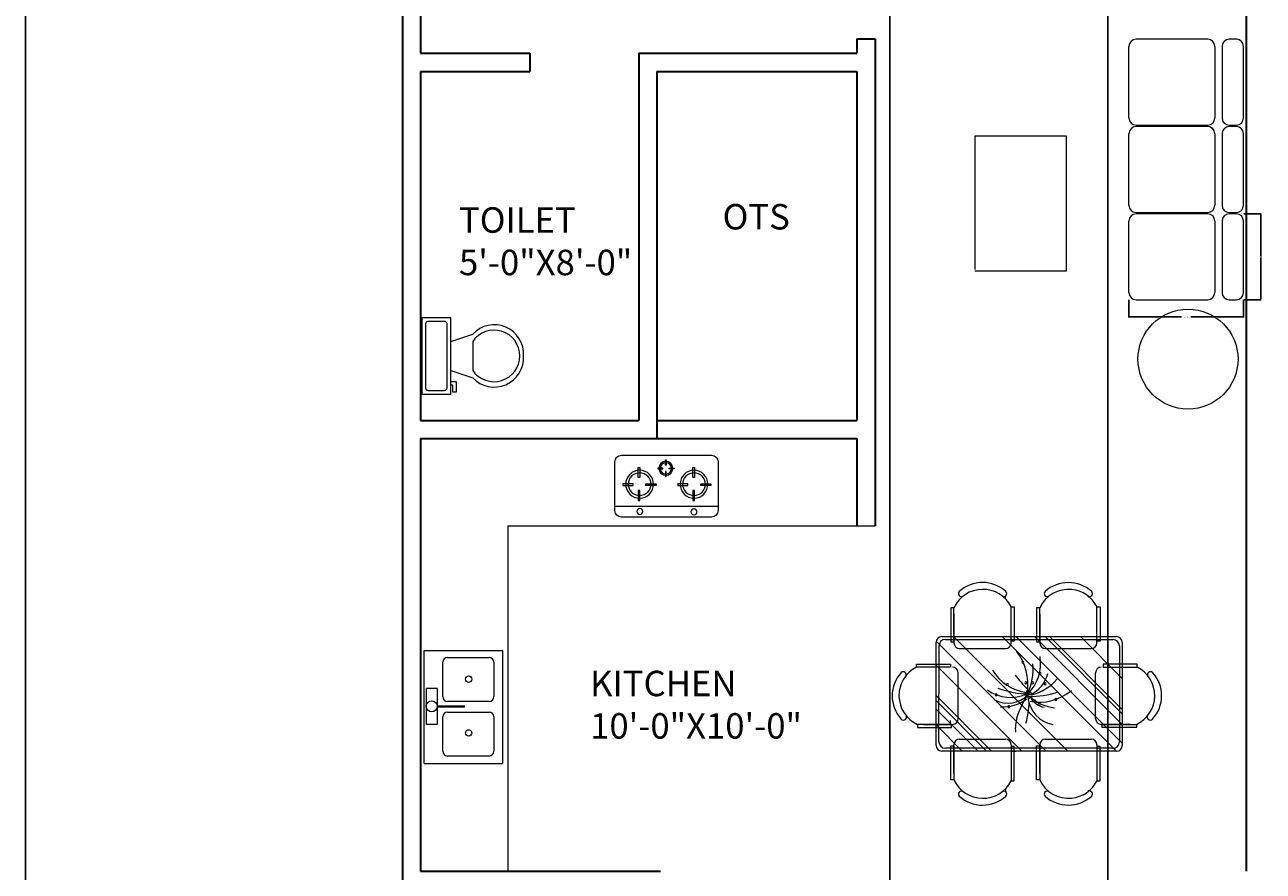
# Model space of a CAD drawing. Units: inches. Extents: x 3731 to 4318, y 1310 to 2388.
# Tile 23 of 57: x 3731 to 4072, y 1554 to 1787. Entities that reach past the tile are written whole.
import ezdxf

# ---------------------------------------------------------------- set-up
doc = ezdxf.new("R2010")
doc.units = ezdxf.units.IN
for name, color, linetype, lineweight in [('A-ANNO-DIMS', 2, 'Continuous', 18), ('A-AREA-IDEN', 7, 'Continuous', 18), ('A-EQPM', 8, 'Continuous', 18), ('A-FLOR-CASE', 8, 'Continuous', 18), ('A-FLOR-FIXT', 9, 'Continuous', 18), ('A-FURN', 8, 'Continuous', 13), ('A-WALL', 7, 'Continuous', 35)]:
    doc.layers.add(name, color=color, linetype=linetype, lineweight=lineweight)
doc.styles.get("Standard").update_dxf_attribs({"font": 'arial.ttf'})
doc.dimstyles.get("Standard").update_dxf_attribs({"dimtxt": 0.18, "dimasz": 0.18, "dimexe": 0.18, "dimexo": 0.0625, "dimgap": 0.09, "dimtad": 0, "dimtih": 1, "dimtoh": 1, "dimdec": 4, "dimzin": 0, "dimdsep": 46, "dimtxsty": 'Standard', "dimcen": 0.09, "dimadec": 0, "dimazin": 0, "dimtfac": 1, "dimtdec": 4, "dimtofl": 0, "dimtmove": 0, "dimatfit": 3, "dimfxl": 1, "dimtolj": 1, "dimtzin": 0, "dimarcsym": 0})

# ---------------------------------------------------------------- blocks, each defined once
blk = doc.blocks.new('A$C6327331B')
for p, q in [((790.8, 678.3), (790.8, 696.4)), ((790.8, 678.3), (790.8, 696.4)), ((1381.3, 692.8), (1381.3, 686.2)), ((1381.3, 692.8), (1381.3, 686.2)), ((410.1, 615.8), (410, 377)), ((410.1, 615.8), (410, 377)), ((431.6, 615.8), (410.1, 615.8)), ((431.6, 615.8), (410.1, 615.8)), ((431.4, 376.9), (431.6, 615.8)), ((431.4, 376.9), (431.6, 615.8)), ((831.4, 382.9), (831.6, 621.7)), ((831.4, 382.9), (831.6, 621.7)), ((831.6, 621.7), (853, 621.7)), ((831.6, 621.7), (853, 621.7)), ((853, 621.7), (852.9, 382.9)), ((853, 621.7), (852.9, 382.9)), ((1009.3, 615.5), (1009.2, 376.7)), ((1009.3, 615.5), (1009.2, 376.7)), ((1030.7, 615.5), (1009.3, 615.5)), ((1030.7, 615.5), (1009.3, 615.5)), ((1030.6, 376.6), (1030.7, 615.5)), ((1030.6, 376.6), (1030.7, 615.5)), ((1430.6, 382.6), (1430.7, 621.4)), ((1430.6, 382.6), (1430.7, 621.4)), ((1430.7, 621.4), (1452.2, 621.4)), ((1430.7, 621.4), (1452.2, 621.4)), ((1452.2, 621.4), (1452, 382.6)), ((1452.2, 621.4), (1452, 382.6)), ((431.5, 571.8), (431.4, 370.8)), ((431.5, 571.8), (431.4, 370.8)), ((831.4, 370.6), (831.5, 571.6)), ((831.4, 370.6), (831.5, 571.6)), ((1030.7, 571.5), (1030.6, 370.5)), ((1030.7, 571.5), (1030.6, 370.5)), ((1430.6, 370.3), (1430.7, 571.3)), ((1430.6, 370.3), (1430.7, 571.3)), ((307.1, -346), (307.5, 374)), ((307.1, -346), (307.5, 374)), ((1075.9, -386.3), (308.5, 383.1)), ((1075.9, -386.3), (308.5, 383.1)), ((327.1, -321), (327.5, 349)), ((347.5, 414), (831.5, 413.8)), ((347.5, 414), (831.5, 413.8)), ((372.5, 394), (831.4, 393.8)), ((372.5, 394), (1009.2, 393.7)), ((410, 377), (431.4, 376.9)), ((410, 377), (431.4, 376.9)), ((1226.3, -386.4), (428, 414)), ((1226.3, -386.4), (428, 414)), ((1567.1, -386.6), (768.8, 413.8)), ((1567.1, -386.6), (768.8, 413.8)), ((852.9, 382.9), (831.4, 382.9)), ((852.9, 382.9), (831.4, 382.9)), ((831.5, 413.8), (1567.5, 413.4)), ((1607.1, -331.3), (864.1, 413.8)), ((1607.1, -331.3), (864.1, 413.8)), ((1607.2, -200.8), (994.4, 413.7)), ((1607.2, -200.8), (994.4, 413.7)), ((1009.2, 413.7), (1567.5, 413.4)), ((1009.2, 393.7), (1542.5, 393.4)), ((1009.2, 376.7), (1030.6, 376.6)), ((1009.2, 376.7), (1030.6, 376.6)), ((1607.2, -125.5), (1069.5, 413.7)), ((1607.2, -125.5), (1069.5, 413.7)), ((1607.2, -95.4), (1099.6, 413.6)), ((1607.2, -95.4), (1099.6, 413.6)), ((1607.3, 120.5), (1315.1, 413.5)), ((1607.3, 120.5), (1315.1, 413.5)), ((1415.7, 413.4), (1415.7, 413.5)), ((1415.7, 413.4), (1415.7, 413.5)), ((1452, 382.6), (1430.6, 382.6)), ((1452, 382.6), (1430.6, 382.6)), ((1587.5, 348.4), (1587.1, -321.6)), ((1607.5, 373.4), (1607.1, -346.6)), ((1607.5, 373.4), (1607.1, -346.6)), ((471.4, 330.8), (791.4, 330.6)), ((471.4, 330.8), (791.4, 330.6)), ((1070.6, 330.5), (1390.6, 330.3)), ((1070.6, 330.5), (1390.6, 330.3)), ((169.9, 221.5), (408.7, 221.6)), ((169.9, 221.5), (408.7, 221.6)), ((169.9, 200.1), (169.9, 221.5)), ((169.9, 200.1), (169.9, 221.5)), ((408.7, 200.2), (169.9, 200.1)), ((408.7, 200.2), (169.9, 200.1)), ((905.5, -386.3), (307.4, 213.5)), ((905.5, -386.3), (307.4, 213.5)), ((408.7, 221.6), (408.7, 200.2)), ((408.7, 221.6), (408.7, 200.2)), ((1473.3, 221.6), (1473.3, 200.2)), ((1473.3, 221.6), (1473.3, 200.2)), ((1712.1, 221.5), (1473.3, 221.6)), ((1712.1, 221.5), (1473.3, 221.6)), ((1473.3, 200.2), (1712.1, 200.1)), ((1473.3, 200.2), (1712.1, 200.1)), ((1712.1, 200.1), (1712.1, 221.5)), ((1712.1, 200.1), (1712.1, 221.5)), ((461.2, -159.8), (461, 160.2)), ((461.2, -159.8), (461, 160.2)), ((1420.8, -159.8), (1420.9, 160.2)), ((1420.8, -159.8), (1420.9, 160.2)), ((695.1, -386.2), (307.3, 2.7)), ((695.1, -386.2), (307.3, 2.7)), ((44.6, -20.2), (44.5, -20.1)), ((44.6, -20.2), (44.5, -20.1)), ((660, -386.1), (307.3, -32.5)), ((660, -386.1), (307.3, -32.5)), ((1837.4, -20.2), (1837.5, -20.1)), ((1837.4, -20.2), (1837.5, -20.1)), ((599.8, -386.1), (307.2, -92.7)), ((599.8, -386.1), (307.2, -92.7)), ((408.7, -193.6), (408.7, -172.1)), ((408.7, -193.6), (408.7, -172.1)), ((415.1, -199.8), (176.2, -199.9)), ((415.1, -199.8), (176.2, -199.9)), ((176.2, -199.9), (176.2, -221.3)), ((176.2, -199.9), (176.2, -221.3)), ((176.2, -221.3), (415.1, -221.2)), ((176.2, -221.3), (415.1, -221.2)), ((220.2, -199.9), (421.2, -199.8)), ((220.2, -199.9), (421.2, -199.8)), ((489.6, -386), (307.2, -203.2)), ((489.6, -386), (307.2, -203.2)), ((415.1, -221.2), (415.1, -199.8)), ((415.1, -221.2), (415.1, -199.8)), ((1661.8, -199.9), (1460.8, -199.8)), ((1661.8, -199.9), (1460.8, -199.8)), ((1466.9, -221.2), (1466.9, -199.8)), ((1466.9, -221.2), (1466.9, -199.8)), ((1466.9, -199.8), (1705.7, -199.9)), ((1466.9, -199.8), (1705.7, -199.9)), ((1705.7, -221.3), (1466.9, -221.2)), ((1705.7, -221.3), (1466.9, -221.2)), ((1705.7, -199.9), (1705.7, -221.3)), ((1705.7, -199.9), (1705.7, -221.3)), ((431.5, -543.7), (431.4, -342.7)), ((431.5, -543.7), (431.4, -342.7)), ((471.4, -302.7), (791.4, -302.5)), ((471.4, -302.7), (791.4, -302.5)), ((831.4, -342.5), (831.5, -543.5)), ((831.4, -342.5), (831.5, -543.5)), ((1030.7, -543.4), (1030.6, -342.4)), ((1030.7, -543.4), (1030.6, -342.4)), ((1070.6, -302.4), (1390.6, -302.2)), ((1070.6, -302.4), (1390.6, -302.2)), ((1430.6, -342.2), (1430.7, -543.2)), ((1430.6, -342.2), (1430.7, -543.2)), ((1567.1, -386.6), (347.1, -386)), ((1567.1, -386.6), (347.1, -386)), ((1542.1, -366.6), (372.1, -366)), ((410.1, -587.7), (410, -348.9)), ((410.1, -587.7), (410, -348.9)), ((410, -348.9), (431.4, -348.9)), ((410, -348.9), (431.4, -348.9)), ((431.4, -348.9), (431.6, -587.7)), ((431.4, -348.9), (431.6, -587.7)), ((831.4, -354.8), (831.6, -593.6)), ((831.4, -354.8), (831.6, -593.6)), ((852.9, -354.8), (831.4, -354.8)), ((852.9, -354.8), (831.4, -354.8)), ((831.5, -385.7), (864.1, -385.7)), ((831.5, -385.7), (864.1, -385.7)), ((853, -593.6), (852.9, -354.8)), ((853, -593.6), (852.9, -354.8)), ((1009.2, -348.6), (1030.6, -348.5)), ((1009.2, -348.6), (1030.6, -348.5)), ((1009.3, -587.4), (1009.2, -348.6)), ((1009.3, -587.4), (1009.2, -348.6)), ((1030.6, -348.5), (1030.7, -587.4)), ((1030.6, -348.5), (1030.7, -587.4)), ((1415.7, -385.3), (1415.7, -385.4)), ((1415.7, -385.3), (1415.7, -385.4)), ((1430.6, -354.5), (1430.7, -593.3)), ((1430.6, -354.5), (1430.7, -593.3)), ((1452, -354.5), (1430.6, -354.5)), ((1452, -354.5), (1430.6, -354.5)), ((1452.2, -593.3), (1452, -354.5)), ((1452.2, -593.3), (1452, -354.5)), ((431.6, -587.7), (410.1, -587.7)), ((431.6, -587.7), (410.1, -587.7)), ((831.6, -593.6), (853, -593.6)), ((831.6, -593.6), (853, -593.6)), ((1030.7, -587.4), (1009.3, -587.4)), ((1030.7, -587.4), (1009.3, -587.4)), ((1430.7, -593.3), (1452.2, -593.3)), ((1430.7, -593.3), (1452.2, -593.3)), ((790.8, -650.2), (790.8, -668.4)), ((790.8, -650.2), (790.8, -668.4)), ((1381.3, -664.7), (1381.3, -658.1)), ((1381.3, -664.7), (1381.3, -658.1))]:
    blk.add_line(p, q)
for centre, radius, start, end in [((631.5, 550.5), 241.3, 47.46915, 132.47205), ((631.5, 550.5), 241.3, 47.46915, 132.47205), ((1230.7, 550.2), 241.3, 47.46915, 132.47205), ((1230.7, 550.2), 241.3, 47.46915, 132.47205), ((633, 521.6), 222.4, 26.76564, 154.93691), ((633, 521.6), 222.4, 26.76564, 154.93691), ((484.3, 714.2), 21.2, 137.64965, 300.34124), ((484.3, 714.2), 21.2, 137.64965, 300.34124), ((779, 714), 21.2, 239.59996, 42.29154), ((779, 714), 21.2, 239.59996, 42.29154), ((1232.2, 521.3), 222.4, 84.42654, 154.93691), ((1232.2, 521.3), 222.4, 84.42654, 154.93691), ((1083.4, 713.9), 21.2, 137.64965, 300.34124), ((1083.4, 713.9), 21.2, 137.64965, 300.34124), ((1232.2, 521.3), 222.4, 26.76564, 84.42654), ((1232.2, 521.3), 222.4, 26.76564, 84.42654), ((1378.1, 713.7), 21.2, 239.59996, 42.29154), ((1378.1, 713.7), 21.2, 239.59996, 42.29154), ((347.5, 374), 40, 89.9706, 179.9706), ((347.5, 374), 40, 89.9706, 179.9706), ((372.5, 349), 45, 89.9706, 179.9706), ((471.4, 370.8), 40, 179.9706, 269.9706), ((471.4, 370.8), 40, 179.9706, 269.9706), ((791.4, 370.6), 40, 269.9706, 359.9706), ((791.4, 370.6), 40, 269.9706, 359.9706), ((1070.6, 370.5), 40, 179.9706, 269.9706), ((1070.6, 370.5), 40, 179.9706, 269.9706), ((1390.6, 370.3), 40, 269.9706, 359.9706), ((1390.6, 370.3), 40, 269.9706, 359.9706), ((1542.5, 348.4), 45, 359.9706, 89.9706), ((1567.5, 373.4), 40, 359.9706, 89.9706), ((1567.5, 373.4), 40, 359.9706, 89.9706), ((574.1, 79.9), 374.6, 351.24958, 38.23328), ((737.8, 225), 299.2, 314.48606, 9.37622), ((270.2, 1.6), 222.4, 116.82445, 244.99571), ((270.2, 1.6), 222.4, 116.82445, 244.99571), ((421, 160.2), 40, 0.0294, 90.0294), ((421, 160.2), 40, 0.0294, 90.0294), ((983.2, 350.8), 331, 211.31505, 262.13779), ((912.6, 235.7), 6.91, 0, 180), ((912.6, 235.7), 6.91, 180, 0), ((586.4, 182.9), 398.1, 335.08876, 5.96372), ((1460.9, 160.2), 40, 89.9706, 179.9706), ((1460.9, 160.2), 40, 89.9706, 179.9706), ((1611.7, 1.6), 222.4, 295.00429, 63.17555), ((1611.7, 1.6), 222.4, 295.00429, 63.17555), ((241.3, 0.1), 241.3, 137.52795, 222.53085), ((77.6, 147.4), 21.2, 329.65876, 132.35035), ((77.6, 147.4), 21.2, 329.65876, 132.35035), ((805, 79.9), 6.91, 0, 180), ((2460.3, 1443.6), 2062.1, 219.04877, 222.6799), ((934.8, 91.3), 6.91, 0, 180), ((934.8, 91.3), 6.91, 180, 0), ((873.8, 207.8), 219.3, 294.09558, 346.29534), ((897.1, 334.6), 335.6, 283.04524, 319.77663), ((982.3, 91.3), 6.91, 0, 180), ((982.3, 91.3), 6.91, 180, 0), ((1033, 155.9), 6.91, 0, 180), ((1033, 155.9), 6.91, 180, 0), ((1067.8, 83.7), 6.91, 0, 180), ((1804.4, 147.4), 21.2, 47.64965, 210.34124), ((1804.4, 147.4), 21.2, 47.64965, 210.34124), ((1640.7, 0.1), 241.3, 317.46915, 42.47205), ((1640.7, 0.1), 241.3, 317.46915, 42.47205), ((826.9, 258.5), 270.1, 233.32313, 295.76326), ((725.8, 7.7), 6.91, 0, 180), ((725.8, 7.7), 6.91, 180, 0), ((807.8, 143), 194.5, 242.99086, 315.91017), ((985.1, 750.7), 739.8, 250.5249, 267.82437), ((805, 79.9), 6.91, 180, 0), ((1747.6, -469.5), 933.6, 148.98728, 160.36101), ((931.7, 11.5), 6.91, 0, 180), ((931.7, 11.5), 6.91, 180, 0), ((944.3, 26.7), 6.91, 0, 180), ((944.3, 26.7), 6.91, 180, 0), ((947.5, 3.9), 6.91, 0, 180), ((947.5, 3.9), 6.91, 180, 0), ((970.7, 574.8), 578.8, 268.32856, 288.729), ((966.5, 15.3), 6.91, 0, 180), ((966.5, 15.3), 6.91, 180, 0), ((1030.3, 292.7), 337.4, 258.55155, 310.98153), ((1067.8, 83.7), 6.91, 180, 0), ((776.7, 191.6), 268.2, 265.87406, 306.95584), ((814.5, -75.9), 6.91, 0, 180), ((814.5, -75.9), 6.91, 180, 0), ((392.7, -33), 564.4, 343.85612, 359.11051), ((953.8, -11.3), 6.91, 0, 180), ((953.8, -11.3), 6.91, 180, 0), ((1167.7, 15.7), 221.9, 186.99045, 258.02836), ((1090.6, 62.7), 145.4, 208.89012, 258.45792), ((1166.2, 212.9), 298.2, 228.7581, 263.8624), ((995, -34.1), 6.91, 0, 180), ((995, -34.1), 6.91, 180, 0), ((1026.7, -60.7), 6.91, 0, 180), ((1026.7, -60.7), 6.91, 180, 0), ((1143.8, -26.5), 6.91, 0, 180), ((1143.8, -26.5), 6.91, 180, 0), ((79, -146.7), 22.5, 226.37763, 29.88821), ((79, -146.7), 22.5, 226.37763, 29.88821), ((421.2, -159.8), 40, 270.0294, 0.0294), ((421.2, -159.8), 40, 270.0294, 0.0294), ((1112.9, -226), 252.6, 162.94564, 186.48138), ((1460.8, -159.8), 40, 179.9706, 269.9706), ((1460.8, -159.8), 40, 179.9706, 269.9706), ((1803, -146.7), 22.5, 150.11179, 313.62237), ((1803, -146.7), 22.5, 150.11179, 313.62237), ((347.1, -346), 40, 179.9706, 269.9706), ((347.1, -346), 40, 179.9706, 269.9706), ((372.1, -321), 45, 179.9706, 269.9706), ((471.4, -342.7), 40, 90.0294, 180.0294), ((471.4, -342.7), 40, 90.0294, 180.0294), ((791.4, -342.5), 40, 0.0294, 90.0294), ((791.4, -342.5), 40, 0.0294, 90.0294), ((1070.6, -342.4), 40, 90.0294, 180.0294), ((1070.6, -342.4), 40, 90.0294, 180.0294), ((1390.6, -342.2), 40, 0.0294, 90.0294), ((1390.6, -342.2), 40, 0.0294, 90.0294), ((1542.1, -321.6), 45, 269.9706, 359.9706), ((1567.1, -346.6), 40, 269.9706, 359.9706), ((1567.1, -346.6), 40, 269.9706, 359.9706), ((633, -493.5), 222.4, 205.06309, 333.23436), ((633, -493.5), 222.4, 205.06309, 333.23436), ((1232.2, -493.2), 222.4, 205.06309, 275.57346), ((1232.2, -493.2), 222.4, 205.06309, 275.57346), ((1232.2, -493.2), 222.4, 275.57346, 333.23436), ((1232.2, -493.2), 222.4, 275.57346, 333.23436), ((484.3, -686.1), 21.2, 59.65876, 222.35035), ((484.3, -686.1), 21.2, 59.65876, 222.35035), ((779, -686), 21.2, 317.70846, 120.40004), ((779, -686), 21.2, 317.70846, 120.40004), ((1083.4, -685.8), 21.2, 59.65876, 222.35035), ((1083.4, -685.8), 21.2, 59.65876, 222.35035), ((1378.1, -685.6), 21.2, 317.70846, 120.40004), ((1378.1, -685.6), 21.2, 317.70846, 120.40004), ((631.5, -522.4), 241.3, 227.52795, 312.53085), ((631.5, -522.4), 241.3, 227.52795, 312.53085), ((1230.7, -522.1), 241.3, 227.52795, 312.53085), ((1230.7, -522.1), 241.3, 227.52795, 312.53085)]:
    blk.add_arc(centre, radius, start, end)
at = {"width": 0.8, "flags": 9}
for tag in ['XSIZE', 'YSIZE']:
    blk.add_attdef(tag, (945.2, 11.4), '', height=0.23, rotation=180, dxfattribs=at)
blk = doc.blocks.new('A$C3AD04490')
for p, q in [((0, 641), (0, 0)), ((0, 641), (925, 641)), ((614, 627), (323, 627)), ((323, 627), (323, 532)), ((614, 532), (614, 627)), ((925, 641), (925, 0)), ((323, 532), (614, 532)), ((463, 312), (463, 537)), ((474, 537), (474, 312)), ((62, 111), (62, 451)), ((101, 490), (383, 490)), ((422, 451), (422, 111)), ((509, 111), (509, 451)), ((548, 490), (830, 490)), ((869, 451), (869, 111)), ((463, 311), (474, 311)), ((383, 72), (101, 72)), ((830, 72), (548, 72)), ((925, 0), (0, 0))]:
    blk.add_line(p, q)
for centre, radius in [((469, 581), 45.9), ((251, 278), 26.4), ((691, 278), 26.4)]:
    blk.add_circle(centre, radius)
for centre, start, end in [((101, 451), 90, 180), ((383, 451), 0, 90), ((548, 451), 90, 180), ((830, 451), 0, 90), ((101, 111), 180, 270), ((383, 111), 270, 0), ((548, 111), 180, 270), ((830, 111), 270, 0)]:
    blk.add_arc(centre, 39.1, start, end)
blk = doc.blocks.new('A$C2A3C6842')
for p, q in [((0, 45), (0, 387)), ((45, 432), (675, 432)), ((161.8, 346.9), (173.2, 346.9)), ((161.8, 275.6), (161.8, 346.9)), ((173.2, 346.9), (173.2, 275.6)), ((351.6, 363.3), (351.6, 398.9)), ((351.6, 398.9), (357.3, 398.9)), ((357.3, 363.3), (351.6, 363.3)), ((357.3, 398.9), (357.3, 363.3)), ((544.7, 346.9), (556.1, 346.9)), ((544.7, 275.6), (544.7, 346.9)), ((556.1, 346.9), (556.1, 275.6)), ((720, 387), (720, 45)), ((173.2, 275.6), (161.8, 275.6)), ((298.4, 341.9), (298.4, 336.2)), ((334, 341.9), (298.4, 341.9)), ((298.4, 336.2), (334, 336.2)), ((334, 336.2), (334, 341.9)), ((357.3, 318.8), (351.6, 318.8)), ((351.6, 318.8), (351.6, 283.1)), ((351.6, 283.1), (357.3, 283.1)), ((357.3, 283.1), (357.3, 318.8)), ((378.5, 336.2), (378.5, 341.9)), ((378.5, 341.9), (414.2, 341.9)), ((414.2, 336.2), (378.5, 336.2)), ((414.2, 341.9), (414.2, 336.2)), ((556.1, 275.6), (544.7, 275.6)), ((55.3, 232.9), (55.3, 221.5)), ((126.6, 232.9), (55.3, 232.9)), ((55.3, 221.5), (126.6, 221.5)), ((126.6, 221.5), (126.6, 232.9)), ((173.2, 186.6), (161.8, 186.6)), ((161.8, 186.6), (161.8, 115.3)), ((173.2, 115.3), (173.2, 186.6)), ((215.6, 221.5), (215.6, 232.9)), ((215.6, 232.9), (286.9, 232.9)), ((286.9, 221.5), (215.6, 221.5)), ((286.9, 232.9), (286.9, 221.5)), ((438.2, 232.9), (438.2, 221.5)), ((509.5, 232.9), (438.2, 232.9)), ((438.2, 221.5), (509.5, 221.5)), ((509.5, 221.5), (509.5, 232.9)), ((556.1, 186.6), (544.7, 186.6)), ((544.7, 186.6), (544.7, 115.3)), ((556.1, 115.3), (556.1, 186.6)), ((598.5, 232.9), (669.8, 232.9)), ((598.5, 221.5), (598.5, 232.9)), ((669.8, 221.5), (598.5, 221.5)), ((669.8, 232.9), (669.8, 221.5)), ((161.8, 115.3), (173.2, 115.3)), ((544.7, 115.3), (556.1, 115.3)), ((1.2, 76.7), (719.9, 76.7)), ((675, 0), (45, 0))]:
    blk.add_line(p, q)
at = {"extrusion": (0, -1e-16, -1)}
for centre, major_axis, start_param, end_param in [((45, 387), (31.8, 31.8), 3.926991, 5.497787), ((172.2, 229.8), (-97.3, 0.1), -0.001099, 6.282086), ((551.8, 229.8), (-97.3, 0.1), -0.001099, 6.282086), ((173.7, 39), (-14.8, 14.8), 5.497787, 11.780972)]:
    blk.add_ellipse(centre, major_axis=major_axis, ratio=1, start_param=start_param, end_param=end_param, dxfattribs=at)
at = {"extrusion": (-1e-16, -1e-16, -1)}
blk.add_ellipse((355.1, 340.4), major_axis=(48.7, 0.1), ratio=1, start_param=3.144125, end_param=9.42731, dxfattribs=at)
at = {"extrusion": (-1e-16, 0, -1)}
for centre, major_axis, start_param, end_param in [((355.1, 340.4), (-39.7, 0), -0.000334, 6.282851), ((45, 45), (-31.8, 31.8), 3.926991, 5.497787)]:
    blk.add_ellipse(centre, major_axis=major_axis, ratio=1, start_param=start_param, end_param=end_param, dxfattribs=at)
at = {"extrusion": (0, 1e-16, -1)}
blk.add_ellipse((675, 387), major_axis=(-31.8, 31.8), ratio=1, start_param=0.785398, end_param=2.356194, dxfattribs=at)
at = {"extrusion": (-1e-16, -4e-16, -1)}
for centre in [(172.2, 229.8), (551.8, 229.8)]:
    blk.add_ellipse(centre, major_axis=(-79.3, 0), ratio=1, start_param=-0.0002116186602152, end_param=6.282973688519371, dxfattribs=at)
at = {"extrusion": (2e-16, -2e-16, -1)}
blk.add_ellipse((551.4, 36.4), major_axis=(14.8, 14.8), ratio=1, start_param=3.926991, end_param=10.210176, dxfattribs=at)
at = {"extrusion": (-2e-16, 1e-16, -1)}
blk.add_ellipse((675, 45), major_axis=(31.8, 31.8), ratio=1, start_param=0.785398, end_param=2.356194, dxfattribs=at)
at = {"text_generation_flag": 4, "flags": 9}
for tag in ['XSIZE', 'YSIZE']:
    blk.add_attdef(tag, (361.3, 264.9), '', height=0.45, rotation=180, dxfattribs=at)
blk = doc.blocks.new('*U14')
for p, q in [((9.5, -6), (9.5, -2)), ((-10, -8.5), (-8, -8.5)), ((-10, -9.5), (-10, -8.5)), ((-7, -9.5), (-10, -9.5)), ((-8, -8.5), (-8, -8)), ((-7, -8), (-7, -9.5)), ((-4, -8), (-6, -14)), ((4, -8), (6, -14)), ((4, -14), (-4, -14))]:
    blk.add_line(p, q)
blk.add_lwpolyline([(10.5, -8), (10.5, 0), (-10.5, 0), (-10.5, -8)], close=True)
for points in [[(-9.5, -2), (-9.5, -6)], [(8.5, -1), (-8.5, -1)], [(-8.5, -7), (8.5, -7)]]:
    blk.add_lwpolyline(points)
for centre, radius, start, end in [((-8.625, -1.875), 0.8839, 81.8699, 188.1301), ((8.625, -1.875), 0.8839, 351.8699, 98.1301), ((-8.625, -6.125), 0.8839, 171.869898, 278.1301), ((8.625, -6.125), 0.8839, 261.8699, 8.1301), ((-0.4772, -19.9188), 8.0953, 133.01722, 273.38), ((0.0374, -19.8731), 7.127, 124.50543, 269.7), ((-0.0373, -19.8731), 7.127, 270.3, 55.4946), ((0.4773, -19.9188), 8.0953, 266.62, 46.9828)]:
    blk.add_arc(centre, radius, start, end)
blk = doc.blocks.new('SOFA-SEAT-MODULE')
for p, q in [((0, 15.22), (0, 21.65)), ((21.65, 23.62), (1.97, 23.62)), ((23.62, 21.65), (23.62, 1.97)), ((25.59, 21.65), (25.59, 1.97)), ((29.53, 23.62), (27.56, 23.62)), ((31.5, 1.97), (31.5, 21.65)), ((0, 1.97), (0, 16.82)), ((1.97, 0), (21.65, 0)), ((27.56, 0), (29.53, 0))]:
    blk.add_line(p, q)
for centre, start, end in [((1.97, 21.65), 90, 180), ((21.65, 21.65), 360, 90), ((21.65, 21.65), 360, 90), ((27.56, 21.65), 90, 180), ((27.56, 21.65), 90, 180), ((29.53, 21.65), 360, 90), ((29.53, 21.65), 360, 90), ((1.97, 1.97), 180, 270), ((21.65, 1.97), 270, 360), ((27.56, 1.97), 180, 270), ((29.53, 1.97), 270, 360)]:
    blk.add_arc(centre, 1.97, start, end)
blk = doc.blocks.new('*D18')
at = {"layer": 'A-ANNO-DIMS', "color": 0, "lineweight": -2, "transparency": 16777216}
for p, q in [((4034.98, 1711.52), (4034.98, 1706.67)), ((4066.48, 1711.52), (4066.48, 1706.67)), ((4035.16, 1706.85), (4049.46, 1706.85)), ((4066.3, 1706.85), (4052, 1706.85))]:
    blk.add_line(p, q, dxfattribs=at)
at = {"layer": 'A-ANNO-DIMS', "color": 0, "transparency": 16777216}
for points in [[(4035.16, 1706.88), (4035.16, 1706.82), (4034.98, 1706.85)], [(4066.3, 1706.88), (4066.3, 1706.82), (4066.48, 1706.85)]]:
    blk.add_solid(points, dxfattribs=at)
at = {"layer": 'Defpoints', "color": 0, "transparency": 16777216}
for p in [(4034.98, 1711.58), (4066.48, 1711.58), (4066.48, 1706.85)]:
    blk.add_point(p, dxfattribs=at)
at = {"layer": 'A-ANNO-DIMS', "color": 0, "transparency": 16777216, "insert": (4050.73, 1706.85), "char_height": 0.18, "attachment_point": 5}
blk.add_mtext('\\A1;SOFA SEAT 31 TYP.', dxfattribs=at)
blk = doc.blocks.new('*D19')
at = {"layer": 'A-ANNO-DIMS', "color": 0, "lineweight": -2, "transparency": 16777216}
for p, q in [((4066.54, 1735.2), (4071.38, 1735.2)), ((4071.2, 1735.02), (4071.2, 1723.57)), ((4071.2, 1711.76), (4071.2, 1723.21)), ((4066.54, 1711.58), (4071.38, 1711.58))]:
    blk.add_line(p, q, dxfattribs=at)
at = {"layer": 'A-ANNO-DIMS', "color": 0, "transparency": 16777216}
for points in [[(4071.17, 1735.02), (4071.23, 1735.02), (4071.2, 1735.2)], [(4071.17, 1711.76), (4071.23, 1711.76), (4071.2, 1711.58)]]:
    blk.add_solid(points, dxfattribs=at)
at = {"layer": 'Defpoints', "color": 0, "transparency": 16777216}
for p in [(4066.48, 1735.2), (4071.2, 1735.2), (4066.48, 1711.58)]:
    blk.add_point(p, dxfattribs=at)
at = {"layer": 'A-ANNO-DIMS', "color": 0, "transparency": 16777216, "insert": (4071.2, 1723.39), "char_height": 0.18, "attachment_point": 5}
blk.add_mtext('\\A1;24 TYP.', dxfattribs=at)
blk = doc.blocks.new('*D32')
at = {"layer": 'A-ANNO-DIMS', "color": 0, "lineweight": -2, "transparency": 16777216}
for p, q in [((4269.21, 1592.32), (4269.21, 1310.25)), ((3835.21, 1359.32), (3835.21, 1310.25)), ((3835.39, 1310.43), (4051.92, 1310.43)), ((4269.03, 1310.43), (4052.5, 1310.43))]:
    blk.add_line(p, q, dxfattribs=at)
at = {"layer": 'A-ANNO-DIMS', "color": 0, "transparency": 16777216}
for points in [[(3835.39, 1310.46), (3835.39, 1310.4), (3835.21, 1310.43)], [(4269.03, 1310.46), (4269.03, 1310.4), (4269.21, 1310.43)]]:
    blk.add_solid(points, dxfattribs=at)
at = {"layer": 'Defpoints', "color": 0, "transparency": 16777216}
for p in [(4269.21, 1592.38), (3835.21, 1359.38), (4269.21, 1310.43)]:
    blk.add_point(p, dxfattribs=at)
at = {"layer": 'A-ANNO-DIMS', "color": 0, "transparency": 16777216, "insert": (4052.21, 1310.43), "char_height": 0.18, "attachment_point": 5}
blk.add_mtext('\\A1;434', dxfattribs=at)
blk = doc.blocks.new('*D33')
at = {"layer": 'A-ANNO-DIMS', "color": 0, "lineweight": -2, "transparency": 16777216}
for p, q in [((3835.15, 2338.38), (3731.41, 2338.38)), ((3731.59, 2338.2), (3731.59, 1849.06)), ((3731.59, 1359.56), (3731.59, 1848.7)), ((3835.15, 1359.38), (3731.41, 1359.38))]:
    blk.add_line(p, q, dxfattribs=at)
at = {"layer": 'A-ANNO-DIMS', "color": 0, "transparency": 16777216}
for points in [[(3731.56, 2338.2), (3731.62, 2338.2), (3731.59, 2338.38)], [(3731.56, 1359.56), (3731.62, 1359.56), (3731.59, 1359.38)]]:
    blk.add_solid(points, dxfattribs=at)
at = {"layer": 'Defpoints', "color": 0, "transparency": 16777216}
for p in [(3731.59, 2338.38), (3835.21, 2338.38), (3835.21, 1359.38)]:
    blk.add_point(p, dxfattribs=at)
at = {"layer": 'A-ANNO-DIMS', "color": 0, "transparency": 16777216, "insert": (3731.59, 1848.88), "char_height": 0.18, "attachment_point": 5}
blk.add_mtext('\\A1;979', dxfattribs=at)
blk = doc.blocks.new('*D44')
at = {"layer": 'A-ANNO-DIMS', "color": 0, "lineweight": -2, "transparency": 16777216}
for p, q in [((3969.21, 1874.32), (3969.21, 1310.25)), ((4029.21, 1874.32), (4029.21, 1310.25)), ((3969.39, 1310.43), (3998.99, 1310.43)), ((4029.03, 1310.43), (3999.43, 1310.43))]:
    blk.add_line(p, q, dxfattribs=at)
at = {"layer": 'A-ANNO-DIMS', "color": 0, "transparency": 16777216}
for points in [[(3969.39, 1310.46), (3969.39, 1310.4), (3969.21, 1310.43)], [(4029.03, 1310.46), (4029.03, 1310.4), (4029.21, 1310.43)]]:
    blk.add_solid(points, dxfattribs=at)
at = {"layer": 'Defpoints', "color": 0, "transparency": 16777216}
for p in [(3969.21, 1874.38), (4029.21, 1874.38), (4029.21, 1310.43)]:
    blk.add_point(p, dxfattribs=at)
at = {"layer": 'A-ANNO-DIMS', "color": 0, "transparency": 16777216, "insert": (3999.21, 1310.43), "char_height": 0.18, "attachment_point": 5}
blk.add_mtext('\\A1;60', dxfattribs=at)

msp = doc.modelspace()

# ---------------------------------------------------------------- linework, layer by layer
at = {"layer": 'A-FLOR-CASE'}
for q in [(3864.21, 1554.38), (3965.21, 1649.38)]:
    msp.add_line((3864.21, 1649.38), q, dxfattribs=at)
at = {"layer": 'A-FURN'}
for p, q in [((4017.83, 1756.54), (3992.64, 1756.54)), ((3992.64, 1756.54), (3992.64, 1719.93)), ((4017.83, 1719.53), (4017.83, 1756.54)), ((3992.64, 1719.53), (4017.83, 1719.53))]:
    msp.add_line(p, q, dxfattribs=at)
msp.add_circle((4051.22, 1695.24), 13.75, dxfattribs=at)
at = {"layer": 'A-WALL'}
for p, q in [((3835.21, 2338.38), (3835.21, 1359.38)), ((3840.21, 1938.38), (3840.21, 1779.38)), ((4067.21, 1803.38), (4067.21, 1554.38)), ((3960.21, 1783.38), (3965.21, 1783.38)), ((3960.21, 1783.38), (3960.21, 1779.38)), ((3965.21, 1783.38), (3965.21, 1779.38)), ((3840.21, 1779.38), (3870.21, 1779.38)), ((3870.21, 1779.38), (3870.21, 1774.38)), ((3900.21, 1779.38), (3900.21, 1678.38)), ((3900.21, 1779.38), (3960.21, 1779.38)), ((3965.21, 1779.38), (3965.21, 1649.38)), ((3840.21, 1774.38), (3870.21, 1774.38)), ((3840.21, 1774.38), (3840.21, 1678.38)), ((3905.21, 1774.38), (3905.21, 1673.38)), ((3905.21, 1774.38), (3960.21, 1774.38)), ((3960.21, 1774.38), (3960.21, 1678.38)), ((3840.21, 1678.38), (3900.21, 1678.38)), ((3905.21, 1678.38), (3960.21, 1678.38)), ((3840.21, 1673.38), (3960.21, 1673.38)), ((3840.21, 1673.38), (3840.21, 1554.38)), ((3960.21, 1673.38), (3960.21, 1649.38)), ((3840.21, 1554.38), (3906.21, 1554.38))]:
    msp.add_line(p, q, dxfattribs=at)

# ---------------------------------------------------------------- block references
at = {"layer": 'A-EQPM', "xscale": 0.0393700787401575, "yscale": 0.0393700787401575, "zscale": 0.0393700787401575}
msp.add_blockref('A$C2A3C6842', (3893.67, 1651.8), dxfattribs=at)
at = {"layer": 'A-FLOR-FIXT', "rotation": 90}
msp.add_blockref('*U14', (3840.54, 1696.13), dxfattribs=at)
at = {"layer": 'A-FLOR-FIXT', "xscale": 0.0336022830821591, "yscale": 0.0336022830821591, "zscale": 0.0336022830821591, "rotation": 90}
msp.add_blockref('A$C3AD04490', (3862.78, 1583.99), dxfattribs=at)
at = {"layer": 'A-FURN'}
for p in [(4034.98, 1759.61), (4034.98, 1735.59), (4034.98, 1711.58)]:
    msp.add_blockref('SOFA-SEAT-MODULE', p, dxfattribs=at)
at = {"layer": 'A-FURN', "xscale": 0.0393700787401575, "yscale": 0.0393700787401575, "zscale": 0.0393700787401575}
msp.add_blockref('A$C6327331B', (3969.87, 1602.63), dxfattribs=at)

# ---------------------------------------------------------------- texts
at = {"layer": 'A-AREA-IDEN', "char_height": 7, "attachment_point": 1}
for s, insert in [('TOILET\\P5\'-0"X8\'-0"', (3850.77, 1737.01)), ('OTS', (3923.26, 1737.91)), ('KITCHEN\\P10\'-0"X10\'-0"', (3886.83, 1609.53))]:
    msp.add_mtext_dynamic_manual_height_columns(s, width=47.0437, gutter_width=12.5, heights=[0], dxfattribs=dict(at, insert=insert))

# ---------------------------------------------------------------- dimensions: what is measured, and where the dimension line sits
at = {"layer": 'A-ANNO-DIMS'}
dim = msp.add_linear_dim(base=(3731.59, 2338.38), p1=(3835.21, 1359.38), p2=(3835.21, 2338.38), angle=90, dimstyle='Standard', override={"dimdec": 0, "dimlfac": 1, "dimrnd": 0, "dimzin": 0, "dimdsep": 46, "dimlunit": 2}, dxfattribs=at)
dim.commit()
dim.dimension.update_dxf_attribs({"geometry": '*D33', "text_midpoint": (3731.59, 1848.88)})
for base, p1, p2, picture, middle in [((4029.21, 1310.43), (3969.21, 1874.38), (4029.21, 1874.38), '*D44', (3999.21, 1310.43)), ((4269.21, 1310.43), (3835.21, 1359.38), (4269.21, 1592.38), '*D32', (4052.21, 1310.43))]:
    dim = msp.add_linear_dim(base=base, p1=p1, p2=p2, dimstyle='Standard', override={"dimdec": 0, "dimlfac": 1, "dimrnd": 0, "dimzin": 0, "dimdsep": 46, "dimlunit": 2}, dxfattribs=at)
    dim.commit()
    dim.dimension.update_dxf_attribs({"geometry": picture, "text_midpoint": middle})
dim = msp.add_linear_dim(base=(4071.2, 1735.2), p1=(4066.48, 1711.58), p2=(4066.48, 1735.2), angle=90, text='<> TYP.', dimstyle='Standard', override={"dimdec": 0, "dimlfac": 1, "dimrnd": 0, "dimzin": 0, "dimdsep": 46, "dimlunit": 2}, dxfattribs=at)
dim.commit()
dim.dimension.update_dxf_attribs({"geometry": '*D19', "text_midpoint": (4071.2, 1723.39)})
dim = msp.add_linear_dim(base=(4066.4796, 1706.8541), p1=(4034.9836, 1711.5785), p2=(4066.4796, 1711.5785), text='SOFA SEAT <> TYP.', dimstyle='Standard', override={"dimdec": 0, "dimlfac": 1, "dimrnd": 0, "dimzin": 0, "dimdsep": 46, "dimlunit": 2}, dxfattribs=at)
dim.commit()
dim.dimension.update_dxf_attribs({"geometry": '*D18', "text_midpoint": (4050.7316, 1706.8541)})

doc.saveas('drawing.dxf')
